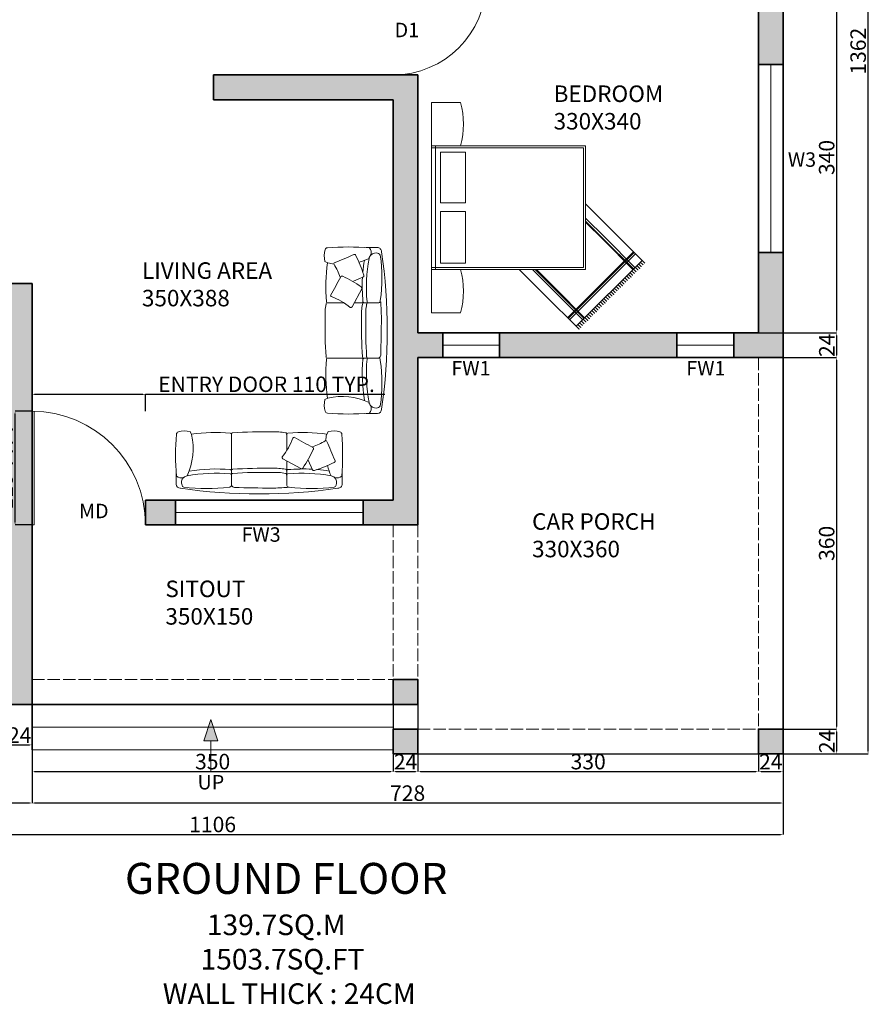
# Model space of a CAD drawing. Units: centimetres. Extents: x 2449 to 7478, y 778 to 2486.
# Tile 2 of 9: x 3072 to 3897, y 778 to 1732. Entities that reach past the tile are written whole.
import ezdxf

# ---------------------------------------------------------------- set-up
doc = ezdxf.new("R2010")
doc.units = ezdxf.units.CM
doc.linetypes.add('ACAD_ISO02W100', pattern=[15, 12, -3])
for name, color, linetype, lineweight in [('A-ANNO-DIMS', 2, 'Continuous', 18), ('A-ANNO-SYMB', 8, 'Continuous', 18), ('A-ANNO-TEXT', 7, 'Continuous', 18), ('A-ANNO-TITL', 7, 'Continuous', 25), ('A-AREA-IDEN', 7, 'Continuous', 18), ('A-COLS', 7, 'Continuous', 35), ('A-COLS-PATT', 7, 'Continuous', 13), ('A-DOOR', 4, 'Continuous', 18), ('A-FLOR', 7, 'Continuous', 25), ('A-FLOR-OVHD', 8, 'ACAD_ISO02W100', 18), ('A-FLOR-STRS', 7, 'Continuous', 18), ('A-WALL', 7, 'Continuous', 35), ('A-WALL-PATT', 7, 'Continuous', 13), ('B-FURNITURE', 22, 'Continuous', 18), ('Win', 1, 'Continuous', 18)]:
    doc.layers.add(name, color=color, linetype=linetype, lineweight=lineweight)
doc.styles.get("Standard").update_dxf_attribs({"font": 'arial.ttf'})
doc.dimstyles.new('ISO-25', dxfattribs={"dimtxt": 15, "dimasz": 2.5, "dimexe": 0, "dimexo": 0, "dimgap": 0, "dimtad": 1, "dimtxsty": 'Standard', "dimcen": 2.5, "dimadec": 0, "dimazin": 0, "dimtfac": 1, "dimtmove": 0, "dimatfit": 3, "dimfxl": 1, "dimarcsym": 0})

# ---------------------------------------------------------------- blocks, each defined once
blk = doc.blocks.new('ролар')
at = {"layer": 'B-FURNITURE'}
for p, q in [((182149, -12928), (182149, -13090)), ((182946, -12908), (182946, -13070)), ((183742, -12908), (183742, -13070)), ((184538, -12927), (184538, -13090)), ((182946, -13070), (182946, -13655)), ((183742, -13070), (183742, -13261)), ((183742, -13412), (183742, -13655))]:
    blk.add_line(p, q, dxfattribs=at)
blk.add_lwpolyline([(184124, -13426, 0.039108), (183972, -13160, 0.352413), (183942, -13151), (183685, -13293, 0.370087), (183675, -13320, -0.085318), (183831, -13592, 0.338149), (183848, -13604, -0.006963), (184118, -13456, 0.478074)], format="xyb", close=True, dxfattribs=at)
blk.add_lwpolyline([(184112, -13464, -0.054969), (184295, -13552, 0.338149), (184316, -13550, -0.006963), (184437, -13268, 0.478074), (184423, -13240, 0.039108), (184140, -13125, 0.352413), (184110, -13136), (184052, -13272)], format="xyb", dxfattribs=at)
for centre, radius, start, end in [((182209, -12928), 60, 90, 180), ((183344, -20690), 7904, 81.7476, 98.2524), ((182264, -12914), 28.1, 104.7154, 176.7534), ((182585, -15161), 2298, 81.7903, 98.2097), ((182918, -12915), 28.9, 15.2961, 99.1888), ((182999, -12942), 63.3, 99.7658, 147.0241), ((181568, 80195), 93085, 270.87421, 271.20678), ((183296, -20822), 7955, 86.6979, 88.3256), ((183770, -12915), 28.9, 80.8112, 164.7039), ((184102, -15161), 2298, 81.7903, 98.2097), ((184423, -12914), 28.1, 3.2466, 75.2846), ((184478, -12928), 60, 358.6006, 89.9879), ((182224, -13128), 110, 72.3508, 130.321), ((182322, -12954), 95.7, 154.4132, 226.8965), ((182340, -12922), 131, 230.7956, 255.727), ((184348, -12922), 131, 284.273, 309.2044), ((184365, -12954), 95.7, 313.1035, 25.5868), ((184464, -13128), 110, 49.679, 107.6492), ((186046, -13346), 3905, 175.5762, 184.4238), ((181452, -13440), 941, 347.608, 24.5904), ((182727, -10699), 2387, 259.8888, 274.8671), ((182725, -10712), 2434, 260.7796, 274.8194), ((182927, -13057), 20.3, 275.8765, 1.8), ((182927, -13117), 20.3, 275.8765, 1.8), ((182962, -13065), 17.3, 149.88, 272.0041), ((182962, -13125), 17.3, 149.88, 272.0041), ((183401, -6361), 6736, 266.2761, 271.089), ((183401, -6421), 6736, 266.2761, 271.089), ((183573, -12278), 819, 266.8813, 280.6931), ((183573, -12338), 819, 266.8813, 280.6931), ((183725, -13065), 17.3, 267.9959, 30.12), ((183725, -13125), 17.3, 267.9959, 30.12), ((183760, -13057), 20.3, 178.2, 264.1235), ((183760, -13117), 20.3, 178.2, 264.1235), ((183961, -10699), 2387, 265.1329, 280.1112), ((184001, -9721), 3425, 265.9379, 271.7664), ((184034, -11509), 1637, 275.2593, 281.2487), ((185235, -13440), 941, 155.4096, 164.8885), ((180641, -13346), 3905, 355.5762, 4.4238), ((185235, -13440), 941, 186.9661, 192.392), ((182195, -13642), 42.7, 187.075, 250.1971), ((182270, -13358), 336, 254.5718, 283.8571), ((181903, -13435), 512, 330.8359, 336.0732), ((182722, -11168), 2503, 261.8987, 274.7524), ((182927, -13643), 20.3, 275.8765, 1.8), ((182962, -13651), 17.3, 149.88, 272.0041), ((183401, -6946), 6736, 266.2761, 271.089), ((183573, -12863), 819, 266.8813, 280.6931), ((183725, -13651), 17.3, 267.9959, 30.12), ((183760, -13643), 20.3, 178.2, 264.1235), ((183966, -11168), 2503, 265.2476, 278.1013), ((184785, -13435), 512, 203.9268, 209.1641), ((184418, -13358), 336, 256.1429, 285.4282), ((184493, -13642), 42.7, 289.8029, 352.925)]:
    blk.add_arc(centre, radius, start, end, dxfattribs=at)
blk = doc.blocks.new('A$C376C2187')
at = {"layer": 'B-FURNITURE'}
for p, q in [((-1.53, 1.82), (-1.53, 2.24)), ((-1.53, 2.24), (-0.9, 2.24)), ((-0.9, 0), (-0.9, 2.24)), ((-0.9, 2.24), (0.9, 2.24)), ((-0.9, 2.24), (-0.9, 1.82)), ((-0.9, 2.182), (0.9, 2.182)), ((-0.87, 0.03), (-0.87, 2.24)), ((0.87, 2.24), (0.87, 0.03)), ((0.9, 2.24), (0.9, 0)), ((0.9, 1.82), (0.9, 2.24)), ((0.9, 2.24), (1.53, 2.24)), ((1.53, 2.24), (1.53, 1.82)), ((-0.807, 2.112), (-0.057, 2.112)), ((-0.807, 1.749), (-0.807, 2.112)), ((-0.057, 2.112), (-0.057, 1.749)), ((0.069, 2.112), (0.807, 2.112)), ((0.069, 2.112), (0.069, 1.749)), ((0.807, 2.112), (0.807, 1.749)), ((-0.807, 1.749), (-0.057, 1.749)), ((0.069, 1.749), (0.807, 1.749)), ((0.9, 0), (-0.9, 0)), ((0.87, 0.03), (-0.87, 0.03))]:
    blk.add_line(p, q, dxfattribs=at)
for centre in [(-1.215, 2.926), (1.215, 2.926)]:
    blk.add_arc(centre, 1.15, 254.0965, 285.9035, dxfattribs=at)
blk = doc.blocks.new('*D41')
at = {"layer": 'A-ANNO-DIMS', "color": 0, "lineweight": -2, "transparency": 16777216}
for p, q in [((3060.09, 1092.34), (3060.09, 1029.04)), ((3084.09, 1068.34), (3084.09, 1029.04)), ((3062.59, 1029.04), (3081.59, 1029.04))]:
    blk.add_line(p, q, dxfattribs=at)
at = {"layer": 'A-ANNO-DIMS', "color": 0, "transparency": 16777216}
for points in [[(3062.59, 1029.46), (3062.59, 1028.62), (3060.09, 1029.04)], [(3081.59, 1029.46), (3081.59, 1028.62), (3084.09, 1029.04)]]:
    blk.add_solid(points, dxfattribs=at)
at = {"layer": 'Defpoints', "color": 0, "transparency": 16777216}
for p in [(3060.09, 1092.34), (3084.09, 1068.34), (3084.09, 1029.04)]:
    blk.add_point(p, dxfattribs=at)
at = {"layer": 'A-ANNO-DIMS', "color": 0, "transparency": 16777216, "insert": (3072.09, 1036.57), "char_height": 15, "attachment_point": 5}
blk.add_mtext('24', dxfattribs=at)
blk = doc.blocks.new('*D42')
at = {"layer": 'A-ANNO-DIMS', "color": 0, "lineweight": -2, "transparency": 16777216}
for p, q in [((3084.09, 1024.34), (3084.09, 1003.23)), ((3434.09, 1020.34), (3434.09, 1003.23)), ((3086.59, 1003.23), (3431.59, 1003.23))]:
    blk.add_line(p, q, dxfattribs=at)
at = {"layer": 'A-ANNO-DIMS', "color": 0, "transparency": 16777216}
for points in [[(3086.59, 1003.64), (3086.59, 1002.81), (3084.09, 1003.23)], [(3431.59, 1003.64), (3431.59, 1002.81), (3434.09, 1003.23)]]:
    blk.add_solid(points, dxfattribs=at)
at = {"layer": 'Defpoints', "color": 0, "transparency": 16777216}
for p in [(3084.09, 1024.34), (3434.09, 1020.34), (3434.09, 1003.23)]:
    blk.add_point(p, dxfattribs=at)
at = {"layer": 'A-ANNO-DIMS', "color": 0, "transparency": 16777216, "insert": (3259.09, 1010.89), "char_height": 15, "attachment_point": 5}
blk.add_mtext('350', dxfattribs=at)
blk = doc.blocks.new('*D43')
at = {"layer": 'A-ANNO-DIMS', "color": 0, "lineweight": -2, "transparency": 16777216}
for p, q in [((3434.09, 1020.34), (3434.09, 1003.23)), ((3458.09, 1020.34), (3458.09, 1003.23)), ((3436.59, 1003.23), (3455.59, 1003.23))]:
    blk.add_line(p, q, dxfattribs=at)
at = {"layer": 'A-ANNO-DIMS', "color": 0, "transparency": 16777216}
for points in [[(3436.59, 1003.64), (3436.59, 1002.81), (3434.09, 1003.23)], [(3455.59, 1003.64), (3455.59, 1002.81), (3458.09, 1003.23)]]:
    blk.add_solid(points, dxfattribs=at)
at = {"layer": 'Defpoints', "color": 0, "transparency": 16777216}
for p in [(3434.09, 1020.34), (3458.09, 1020.34), (3458.09, 1003.23)]:
    blk.add_point(p, dxfattribs=at)
at = {"layer": 'A-ANNO-DIMS', "color": 0, "transparency": 16777216, "insert": (3446.09, 1010.76), "char_height": 15, "attachment_point": 5}
blk.add_mtext('24', dxfattribs=at)
blk = doc.blocks.new('*D44')
at = {"layer": 'A-ANNO-DIMS', "color": 0, "lineweight": -2, "transparency": 16777216}
for p, q in [((3458.09, 1020.34), (3458.09, 1003.23)), ((3788.09, 1020.34), (3788.09, 1003.23)), ((3460.59, 1003.23), (3785.59, 1003.23))]:
    blk.add_line(p, q, dxfattribs=at)
at = {"layer": 'A-ANNO-DIMS', "color": 0, "transparency": 16777216}
for points in [[(3460.59, 1003.64), (3460.59, 1002.81), (3458.09, 1003.23)], [(3785.59, 1003.64), (3785.59, 1002.81), (3788.09, 1003.23)]]:
    blk.add_solid(points, dxfattribs=at)
at = {"layer": 'Defpoints', "color": 0, "transparency": 16777216}
for p in [(3458.09, 1020.34), (3788.09, 1020.34), (3788.09, 1003.23)]:
    blk.add_point(p, dxfattribs=at)
at = {"layer": 'A-ANNO-DIMS', "color": 0, "transparency": 16777216, "insert": (3623.09, 1010.89), "char_height": 15, "attachment_point": 5}
blk.add_mtext('330', dxfattribs=at)
blk = doc.blocks.new('*D45')
at = {"layer": 'A-ANNO-DIMS', "color": 0, "lineweight": -2, "transparency": 16777216}
for p, q in [((3788.09, 1020.34), (3788.09, 1003.23)), ((3812.09, 1020.34), (3812.09, 1003.23)), ((3790.59, 1003.23), (3809.59, 1003.23))]:
    blk.add_line(p, q, dxfattribs=at)
at = {"layer": 'A-ANNO-DIMS', "color": 0, "transparency": 16777216}
for points in [[(3790.59, 1003.64), (3790.59, 1002.81), (3788.09, 1003.23)], [(3809.59, 1003.64), (3809.59, 1002.81), (3812.09, 1003.23)]]:
    blk.add_solid(points, dxfattribs=at)
at = {"layer": 'Defpoints', "color": 0, "transparency": 16777216}
for p in [(3788.09, 1020.34), (3812.09, 1020.34), (3812.09, 1003.23)]:
    blk.add_point(p, dxfattribs=at)
at = {"layer": 'A-ANNO-DIMS', "color": 0, "transparency": 16777216, "insert": (3800.09, 1010.76), "char_height": 15, "attachment_point": 5}
blk.add_mtext('24', dxfattribs=at)
blk = doc.blocks.new('*D51')
at = {"layer": 'A-ANNO-DIMS', "color": 0, "lineweight": -2, "transparency": 16777216}
for p, q in [((3788.09, 1768.34), (3863.83, 1768.34)), ((3863.83, 1765.84), (3863.83, 1430.84)), ((3788.09, 1428.34), (3863.83, 1428.34))]:
    blk.add_line(p, q, dxfattribs=at)
at = {"layer": 'A-ANNO-DIMS', "color": 0, "transparency": 16777216}
for points in [[(3863.42, 1765.84), (3864.25, 1765.84), (3863.83, 1768.34)], [(3863.42, 1430.84), (3864.25, 1430.84), (3863.83, 1428.34)]]:
    blk.add_solid(points, dxfattribs=at)
at = {"layer": 'Defpoints', "color": 0, "transparency": 16777216}
for p in [(3788.09, 1768.34), (3788.09, 1428.34), (3863.83, 1428.34)]:
    blk.add_point(p, dxfattribs=at)
at = {"layer": 'A-ANNO-DIMS', "color": 0, "transparency": 16777216, "insert": (3856.17, 1598.34), "char_height": 15, "attachment_point": 5, "rotation": 90}
blk.add_mtext('340', dxfattribs=at)
blk = doc.blocks.new('*D52')
at = {"layer": 'A-ANNO-DIMS', "color": 0, "lineweight": -2, "transparency": 16777216}
for p, q in [((3788.09, 1428.34), (3863.83, 1428.34)), ((3863.83, 1425.84), (3863.83, 1406.84)), ((3812.09, 1404.34), (3863.83, 1404.34))]:
    blk.add_line(p, q, dxfattribs=at)
at = {"layer": 'A-ANNO-DIMS', "color": 0, "transparency": 16777216}
for points in [[(3863.42, 1425.84), (3864.25, 1425.84), (3863.83, 1428.34)], [(3863.42, 1406.84), (3864.25, 1406.84), (3863.83, 1404.34)]]:
    blk.add_solid(points, dxfattribs=at)
at = {"layer": 'Defpoints', "color": 0, "transparency": 16777216}
for p in [(3788.09, 1428.34), (3812.09, 1404.34), (3863.83, 1404.34)]:
    blk.add_point(p, dxfattribs=at)
at = {"layer": 'A-ANNO-DIMS', "color": 0, "transparency": 16777216, "insert": (3856.3, 1416.34), "char_height": 15, "attachment_point": 5, "rotation": 90}
blk.add_mtext('24', dxfattribs=at)
blk = doc.blocks.new('*D53')
at = {"layer": 'A-ANNO-DIMS', "color": 0, "lineweight": -2, "transparency": 16777216}
for p, q in [((3812.09, 1404.34), (3863.83, 1404.34)), ((3863.83, 1401.84), (3863.83, 1046.84)), ((3812.09, 1044.34), (3863.83, 1044.34))]:
    blk.add_line(p, q, dxfattribs=at)
at = {"layer": 'A-ANNO-DIMS', "color": 0, "transparency": 16777216}
for points in [[(3863.42, 1401.84), (3864.25, 1401.84), (3863.83, 1404.34)], [(3863.42, 1046.84), (3864.25, 1046.84), (3863.83, 1044.34)]]:
    blk.add_solid(points, dxfattribs=at)
at = {"layer": 'Defpoints', "color": 0, "transparency": 16777216}
for p in [(3812.09, 1404.34), (3812.09, 1044.34), (3863.83, 1044.34)]:
    blk.add_point(p, dxfattribs=at)
at = {"layer": 'A-ANNO-DIMS', "color": 0, "transparency": 16777216, "insert": (3856.17, 1224.34), "char_height": 15, "attachment_point": 5, "rotation": 90}
blk.add_mtext('360', dxfattribs=at)
blk = doc.blocks.new('*D54')
at = {"layer": 'A-ANNO-DIMS', "color": 0, "lineweight": -2, "transparency": 16777216}
for p, q in [((3812.09, 1044.34), (3863.83, 1044.34)), ((3863.83, 1041.84), (3863.83, 1022.84)), ((3812.09, 1020.34), (3863.83, 1020.34))]:
    blk.add_line(p, q, dxfattribs=at)
at = {"layer": 'A-ANNO-DIMS', "color": 0, "transparency": 16777216}
for points in [[(3863.42, 1041.84), (3864.25, 1041.84), (3863.83, 1044.34)], [(3863.42, 1022.84), (3864.25, 1022.84), (3863.83, 1020.34)]]:
    blk.add_solid(points, dxfattribs=at)
at = {"layer": 'Defpoints', "color": 0, "transparency": 16777216}
for p in [(3812.09, 1044.34), (3812.09, 1020.34), (3863.83, 1020.34)]:
    blk.add_point(p, dxfattribs=at)
at = {"layer": 'A-ANNO-DIMS', "color": 0, "transparency": 16777216, "insert": (3856.3, 1032.34), "char_height": 15, "attachment_point": 5, "rotation": 90}
blk.add_mtext('24', dxfattribs=at)
blk = doc.blocks.new('*D55')
at = {"layer": 'A-ANNO-DIMS', "color": 0, "lineweight": -2, "transparency": 16777216}
for p, q in [((3084.09, 1068.34), (3084.09, 972.69)), ((3812.09, 1020.34), (3812.09, 972.69)), ((3809.59, 972.69), (3086.59, 972.69))]:
    blk.add_line(p, q, dxfattribs=at)
at = {"layer": 'A-ANNO-DIMS', "color": 0, "transparency": 16777216}
for points in [[(3086.59, 973.11), (3086.59, 972.27), (3084.09, 972.69)], [(3809.59, 973.11), (3809.59, 972.27), (3812.09, 972.69)]]:
    blk.add_solid(points, dxfattribs=at)
at = {"layer": 'Defpoints', "color": 0, "transparency": 16777216}
for p in [(3084.09, 1068.34), (3812.09, 1020.34), (3084.09, 972.69)]:
    blk.add_point(p, dxfattribs=at)
at = {"layer": 'A-ANNO-DIMS', "color": 0, "transparency": 16777216, "insert": (3448.09, 980.35), "char_height": 15, "attachment_point": 5}
blk.add_mtext('728', dxfattribs=at)
blk = doc.blocks.new('*D56')
at = {"layer": 'A-ANNO-DIMS', "color": 0, "lineweight": -2, "transparency": 16777216}
for p, q in [((2706.09, 1068.34), (2706.09, 972.69)), ((3084.09, 1068.34), (3084.09, 972.69)), ((3081.59, 972.69), (2708.59, 972.69))]:
    blk.add_line(p, q, dxfattribs=at)
at = {"layer": 'A-ANNO-DIMS', "color": 0, "transparency": 16777216}
for points in [[(2708.59, 973.11), (2708.59, 972.27), (2706.09, 972.69)], [(3081.59, 973.11), (3081.59, 972.27), (3084.09, 972.69)]]:
    blk.add_solid(points, dxfattribs=at)
at = {"layer": 'Defpoints', "color": 0, "transparency": 16777216}
for p in [(2706.09, 1068.34), (3084.09, 1068.34), (2706.09, 972.69)]:
    blk.add_point(p, dxfattribs=at)
at = {"layer": 'A-ANNO-DIMS', "color": 0, "transparency": 16777216, "insert": (2895.09, 980.35), "char_height": 15, "attachment_point": 5}
blk.add_mtext('378', dxfattribs=at)
blk = doc.blocks.new('*D57')
at = {"layer": 'A-ANNO-DIMS', "color": 0, "lineweight": -2, "transparency": 16777216}
for p, q in [((2706.09, 1068.34), (2706.09, 942.3)), ((3812.09, 1044.34), (3812.09, 942.3)), ((2708.59, 942.3), (3809.59, 942.3))]:
    blk.add_line(p, q, dxfattribs=at)
at = {"layer": 'A-ANNO-DIMS', "color": 0, "transparency": 16777216}
for points in [[(2708.59, 942.72), (2708.59, 941.88), (2706.09, 942.3)], [(3809.59, 942.72), (3809.59, 941.88), (3812.09, 942.3)]]:
    blk.add_solid(points, dxfattribs=at)
at = {"layer": 'Defpoints', "color": 0, "transparency": 16777216}
for p in [(2706.09, 1068.34), (3812.09, 1044.34), (3812.09, 942.3)]:
    blk.add_point(p, dxfattribs=at)
at = {"layer": 'A-ANNO-DIMS', "color": 0, "transparency": 16777216, "insert": (3259.09, 949.96), "char_height": 15, "attachment_point": 5}
blk.add_mtext('1106', dxfattribs=at)
blk = doc.blocks.new('*D58')
at = {"layer": 'A-ANNO-DIMS', "color": 0, "lineweight": -2, "transparency": 16777216}
for p, q in [((3812.09, 2382.34), (3894.34, 2382.34)), ((3894.34, 1022.84), (3894.34, 2379.84)), ((3812.09, 1020.34), (3894.34, 1020.34))]:
    blk.add_line(p, q, dxfattribs=at)
at = {"layer": 'A-ANNO-DIMS', "color": 0, "transparency": 16777216}
for points in [[(3893.92, 2379.84), (3894.76, 2379.84), (3894.34, 2382.34)], [(3893.92, 1022.84), (3894.76, 1022.84), (3894.34, 1020.34)]]:
    blk.add_solid(points, dxfattribs=at)
at = {"layer": 'Defpoints', "color": 0, "transparency": 16777216}
for p in [(3812.09, 2382.34), (3894.34, 2382.34), (3812.09, 1020.34)]:
    blk.add_point(p, dxfattribs=at)
at = {"layer": 'A-ANNO-DIMS', "color": 0, "transparency": 16777216, "insert": (3886.68, 1701.34), "char_height": 15, "attachment_point": 5, "rotation": 90}
blk.add_mtext('1362', dxfattribs=at)
blk = doc.blocks.new('1')
for p, q in [((5854.12, 1703.75), (5854.12, 1593.75)), ((5856.12, 1703.75), (5856.12, 1593.75)), ((5856.12, 1593.75), (5854.12, 1593.75))]:
    blk.add_line(p, q)
blk.add_arc((5854.12, 1593.75), 110, 0, 90)
blk = doc.blocks.new('2')
for p, q in [((5717.35, 1812.71), (5717.35, 1722.71)), ((5719.35, 1812.71), (5719.35, 1722.71)), ((5719.35, 1722.71), (5717.35, 1722.71))]:
    blk.add_line(p, q)
blk.add_arc((5717.35, 1722.71), 90, 0, 90)
blk = doc.blocks.new('RUG-FRINGED-B')
for p, q in [((90.45, 95.22), (64.35, 121.32)), ((64.35, 107.43), (83.5, 88.28)), ((64.35, 104.72), (82.15, 86.92)), ((64.35, 103.56), (81.57, 86.34)), ((110.18, 57.73), (81.57, 86.34)), ((110.76, 58.31), (82.15, 86.92)), ((112.12, 59.66), (83.5, 88.28)), ((90.45, 95.22), (119.07, 66.61)), ((110.74, 74.93), (46.79, 10.99)), ((111.32, 74.35), (47.37, 10.4)), ((112.68, 73), (48.73, 9.05)), ((0, 57.78), (26.5, 31.28)), ((32.89, 37.67), (12.78, 57.78)), ((34.25, 39.02), (15.49, 57.78)), ((34.83, 39.6), (16.65, 57.78)), ((119.07, 66.61), (55.12, 2.66)), ((110.66, 58.21), (113.29, 55.58)), ((112.34, 59.89), (114.97, 57.26)), ((114.02, 61.57), (116.65, 58.94)), ((115.7, 63.25), (118.33, 60.62)), ((117.39, 64.93), (120.01, 62.3)), ((119.07, 66.61), (121.69, 63.98)), ((100.58, 48.13), (103.21, 45.5)), ((102.26, 49.81), (104.89, 47.18)), ((103.94, 51.49), (106.57, 48.86)), ((105.62, 53.17), (108.25, 50.54)), ((107.3, 54.85), (109.93, 52.22)), ((108.98, 56.53), (111.61, 53.9)), ((34.25, 39.02), (62.86, 10.4)), ((34.83, 39.6), (63.44, 10.99)), ((92.18, 39.73), (94.81, 37.1)), ((93.86, 41.41), (96.49, 38.78)), ((95.54, 43.09), (98.17, 40.46)), ((97.22, 44.77), (99.85, 42.14)), ((98.9, 46.45), (101.53, 43.82)), ((55.12, 2.66), (26.5, 31.28)), ((32.89, 37.67), (61.51, 9.05)), ((82.1, 29.65), (84.73, 27.02)), ((83.78, 31.33), (86.41, 28.7)), ((85.46, 33.01), (88.09, 30.38)), ((87.14, 34.69), (89.77, 32.06)), ((88.82, 36.37), (91.45, 33.74)), ((90.5, 38.05), (93.13, 35.42)), ((72.02, 19.57), (74.65, 16.94)), ((73.7, 21.25), (76.33, 18.62)), ((75.38, 22.93), (78.01, 20.3)), ((77.06, 24.61), (79.69, 21.98)), ((78.74, 26.29), (81.37, 23.66)), ((80.42, 27.97), (83.05, 25.34)), ((63.62, 11.17), (66.25, 8.54)), ((65.3, 12.85), (67.93, 10.22)), ((66.98, 14.53), (69.61, 11.9)), ((68.66, 16.21), (71.29, 13.58)), ((70.34, 17.89), (72.97, 15.26)), ((55.22, 2.76), (57.85, 0.14)), ((56.9, 4.44), (59.53, 1.82)), ((58.58, 6.12), (61.21, 3.5)), ((60.26, 7.8), (62.89, 5.18)), ((61.94, 9.48), (64.57, 6.86))]:
    blk.add_line(p, q)
for centre in [(115.03, 57.2), (116.71, 58.88), (118.39, 60.56), (120.07, 62.24), (121.75, 63.92), (106.63, 48.8), (108.31, 50.48), (109.99, 52.16), (111.67, 53.84), (113.35, 55.52), (96.55, 38.72), (98.23, 40.4), (99.91, 42.08), (101.59, 43.76), (103.27, 45.44), (104.95, 47.12), (86.47, 28.64), (88.15, 30.32), (89.83, 32), (91.51, 33.68), (93.19, 35.36), (94.87, 37.04), (78.07, 20.24), (79.75, 21.92), (81.43, 23.6), (83.11, 25.28), (84.79, 26.96), (67.99, 10.16), (69.67, 11.84), (71.35, 13.52), (73.03, 15.2), (74.71, 16.88), (76.39, 18.56), (57.91, 0.08), (59.59, 1.76), (61.27, 3.44), (62.95, 5.12), (64.63, 6.8), (66.31, 8.48)]:
    blk.add_circle(centre, 0.0789)
blk = doc.blocks.new('ARROW-ENTRY-UP')
at = {"transparency": 33554687}
h = blk.add_hatch(color=256, dxfattribs=at)
h.dxf.hatch_style = 1
h.paths.add_polyline_path([(-6.84, 30.34), (6.84, 30.34), (0, 51.25)])
blk.add_line((0, 30.34), (0, 0))
blk.add_lwpolyline([(0, 51.25), (-6.84, 30.34), (6.84, 30.34)], close=True)
blk = doc.blocks.new('*D72')
at = {"layer": 'A-ANNO-DIMS', "color": 0, "lineweight": -2, "transparency": 16777216}
for p, q in [((3084.09, 1352.34), (3084.09, 1368.84)), ((3086.59, 1368.84), (3191.59, 1368.84)), ((3194.09, 1352.34), (3194.09, 1368.84)), ((3194.09, 1368.84), (3426, 1368.84))]:
    blk.add_line(p, q, dxfattribs=at)
at = {"layer": 'A-ANNO-DIMS', "color": 0, "transparency": 16777216}
for points in [[(3086.59, 1369.26), (3086.59, 1368.42), (3084.09, 1368.84)], [(3191.59, 1369.26), (3191.59, 1368.42), (3194.09, 1368.84)]]:
    blk.add_solid(points, dxfattribs=at)
at = {"layer": 'Defpoints', "color": 0, "transparency": 16777216}
for p in [(3194.09, 1368.84), (3084.09, 1352.34), (3194.09, 1352.34)]:
    blk.add_point(p, dxfattribs=at)
at = {"layer": 'A-ANNO-DIMS', "color": 0, "transparency": 16777216, "insert": (3311.29, 1376.6), "char_height": 15, "attachment_point": 5}
blk.add_mtext('ENTRY DOOR 110 TYP.', dxfattribs=at)
blk = doc.blocks.new('*D73')
at = {"layer": 'A-ANNO-DIMS', "color": 0, "lineweight": -2, "transparency": 16777216}
for p, q in [((3084.09, 1352.34), (3067.59, 1352.34)), ((3067.59, 1244.84), (3067.59, 1349.84)), ((3084.09, 1242.34), (3067.59, 1242.34))]:
    blk.add_line(p, q, dxfattribs=at)
at = {"layer": 'A-ANNO-DIMS', "color": 0, "transparency": 16777216}
for points in [[(3067.17, 1349.84), (3068, 1349.84), (3067.59, 1352.34)], [(3067.17, 1244.84), (3068, 1244.84), (3067.59, 1242.34)]]:
    blk.add_solid(points, dxfattribs=at)
at = {"layer": 'Defpoints', "color": 0, "transparency": 16777216}
for p in [(3067.59, 1352.34), (3084.09, 1352.34), (3084.09, 1242.34)]:
    blk.add_point(p, dxfattribs=at)
at = {"layer": 'A-ANNO-DIMS', "color": 0, "transparency": 16777216, "insert": (3059.93, 1297.34), "char_height": 15, "attachment_point": 5, "rotation": 90}
blk.add_mtext('110 TYP.', dxfattribs=at)

msp = doc.modelspace()

# ---------------------------------------------------------------- hatches: boundary and pattern name
at = {"layer": 'A-COLS-PATT'}
h = msp.add_hatch(color=256, dxfattribs=at)
h.dxf.hatch_style = 1
h.paths.add_polyline_path([(3458.088, 1092.34), (3434.088, 1092.34), (3434.088, 1068.34), (3458.088, 1068.34)])
h = msp.add_hatch(color=256, dxfattribs=at)
h.dxf.hatch_style = 1
h.paths.add_polyline_path([(3434.088, 1020.34), (3458.088, 1020.34), (3458.088, 1044.34), (3434.088, 1044.34)])
h = msp.add_hatch(color=256, dxfattribs=at)
h.dxf.hatch_style = 1
h.paths.add_polyline_path([(3788.088, 1020.34), (3812.088, 1020.34), (3812.088, 1044.34), (3788.088, 1044.34)])
at = {"layer": 'A-WALL-PATT'}
h = msp.add_hatch(color=256, dxfattribs=at)
h.dxf.hatch_style = 1
h.paths.add_polyline_path([(3060.088, 1092.34), (2986.088, 1092.34), (2986.088, 1068.34), (3084.088, 1068.34), (3084.088, 1476.34), (3060.088, 1476.34)])
h.paths.add_polyline_path([(2706.088, 1167.34), (2730.088, 1167.34), (2730.088, 1377.34), (2706.088, 1377.34)])
h.paths.add_polyline_path([(2804.088, 1068.34), (2804.088, 1092.34), (2730.088, 1092.34), (2730.088, 1112.34), (2706.088, 1112.34), (2706.088, 1068.34)])
h.paths.add_polyline_path([(2730.088, 1551.34), (2706.088, 1551.34), (2706.088, 1432.34), (2730.088, 1432.34), (2730.088, 1452.34), (2970.088, 1452.34), (2970.088, 1476.34), (2730.088, 1476.34)])
h.paths.add_polyline_path([(3434.088, 1654.34), (3434.088, 1266.34), (3405.088, 1266.34), (3405.088, 1242.34), (3458.088, 1242.34), (3458.088, 1404.34), (3482.088, 1404.34), (3482.088, 1428.34), (3458.088, 1428.34), (3458.088, 1678.34), (3260.088, 1678.34), (3260.088, 1654.34)])
h.paths.add_polyline_path([(3223.088, 1266.34), (3194.088, 1266.34), (3194.088, 1242.34), (3223.088, 1242.34)])
h.paths.add_polyline_path([(3812.088, 1506.339), (3788.088, 1506.339), (3788.088, 1428.34), (3764.088, 1428.34), (3764.088, 1404.34), (3812.088, 1404.34)])
h.paths.add_polyline_path([(3709.088, 1404.34), (3709.088, 1428.34), (3537.088, 1428.34), (3537.088, 1404.34)])
h.paths.add_polyline_path([(3788.088, 1688.339), (3812.088, 1688.339), (3812.088, 1826.34), (3788.088, 1826.34), (3788.088, 1792.34), (3647.088, 1792.34), (3647.088, 1768.34), (3788.088, 1768.34)])
h.paths.add_polyline_path([(3788.088, 1956.34), (3548.088, 1956.34), (3548.088, 1792.34), (3434.088, 1792.34), (3434.088, 1768.34), (3572.088, 1768.34), (3572.088, 1932.34), (3788.088, 1932.34), (3788.088, 1898.34), (3812.088, 1898.34), (3812.088, 2065.339), (3788.088, 2065.339)])
h.paths.add_polyline_path([(3788.088, 2358.34), (3788.088, 2247.339), (3812.088, 2247.339), (3812.088, 2382.34), (3764.088, 2382.34), (3764.088, 2358.34)])
h.paths.add_polyline_path([(3537.088, 2382.34), (3537.088, 2358.34), (3709.088, 2358.34), (3709.088, 2382.34)])
h.paths.add_polyline_path([(3458.088, 2358.34), (3482.088, 2358.34), (3482.088, 2382.34), (3434.088, 2382.34), (3434.088, 2214.34), (3395.088, 2214.34), (3395.088, 2190.34), (3434.088, 2190.34), (3434.088, 2065.34), (3458.088, 2065.34)])
h.paths.add_polyline_path([(3231.088, 2214.34), (3231.088, 2190.34), (3260.088, 2190.34), (3260.088, 1966.34), (3434.088, 1966.34), (3434.088, 1932.34), (3458.088, 1932.34), (3458.088, 1990.34), (3284.088, 1990.34), (3284.088, 2190.34), (3323.088, 2190.34), (3323.088, 2214.34)])
h.paths.add_polyline_path([(3130.088, 2190.34), (3159.088, 2190.34), (3159.088, 2214.34), (3032.088, 2214.34), (3032.088, 2190.34), (3106.088, 2190.34), (3106.088, 1836.34), (3130.088, 1836.34), (3130.088, 1966.34), (3185.088, 1966.34), (3185.088, 1990.34), (3130.088, 1990.34)])
h.paths.add_polyline_path([(2738.088, 2214.34), (2738.088, 2190.34), (2752.088, 2190.34), (2752.088, 1935.34), (2776.088, 1935.34), (2776.088, 2190.34), (2850.088, 2190.34), (2850.088, 2214.34)])
h.paths.add_polyline_path([(2578.088, 2152.839), (2602.088, 2152.839), (2602.088, 2190.34), (2616.088, 2190.34), (2616.088, 2214.34), (2578.088, 2214.34)])
h.paths.add_polyline_path([(2578.088, 1935.34), (2602.088, 1935.34), (2602.088, 1970.839), (2578.088, 1970.839)])
h.paths.add_polyline_path([(2706.088, 1836.34), (2706.088, 1791.34), (2730.088, 1791.34), (2730.088, 1836.34), (3016.088, 1836.34), (3016.088, 1860.34), (2578.088, 1860.34), (2578.088, 1836.34)])

# ---------------------------------------------------------------- linework, layer by layer
at = {"layer": 'A-COLS'}
for points in [[(3434.088, 1068.34), (3458.088, 1068.34), (3458.088, 1092.34), (3434.088, 1092.34)], [(3434.088, 1020.34), (3458.088, 1020.34), (3458.088, 1044.34), (3434.088, 1044.34)], [(3788.088, 1020.34), (3812.088, 1020.34), (3812.088, 1044.34), (3788.088, 1044.34)]]:
    msp.add_lwpolyline(points, close=True, dxfattribs=at)
at = {"layer": 'A-FLOR'}
for p, q in [((3434.088, 1092.34), (3434.088, 1020.34)), ((3458.088, 1092.34), (3458.088, 1044.34)), ((3434.088, 1044.34), (3458.088, 1044.34)), ((3434.088, 1020.34), (3812.088, 1020.34))]:
    msp.add_line(p, q, dxfattribs=at)
at = {"layer": 'A-FLOR-OVHD'}
for p, q in [((3788.088, 1404.34), (3788.088, 1044.34)), ((3434.088, 1242.34), (3434.088, 1092.34)), ((3458.088, 1242.34), (3458.088, 1092.34)), ((3084.088, 1092.34), (3458.088, 1092.34)), ((3458.088, 1044.34), (3788.088, 1044.34))]:
    msp.add_line(p, q, dxfattribs=at)
at = {"layer": 'A-FLOR-STRS'}
for p, q in [((3084.088, 1046.34), (3434.088, 1046.34)), ((3084.088, 1024.34), (3434.088, 1024.34))]:
    msp.add_line(p, q, dxfattribs=at)
at = {"layer": 'A-WALL'}
for p, q in [((3812.088, 2382.34), (3812.088, 1020.34)), ((3788.088, 1768.34), (3788.088, 1428.34)), ((3788.088, 1688.339), (3812.088, 1688.339)), ((3260.088, 1678.34), (3458.088, 1678.34)), ((3260.088, 1678.34), (3260.088, 1654.34)), ((3458.088, 1678.34), (3458.088, 1428.34)), ((3260.088, 1654.34), (3434.088, 1654.34)), ((3434.088, 1654.34), (3434.088, 1266.34)), ((3788.088, 1506.339), (3812.088, 1506.339)), ((3060.088, 1476.34), (3084.088, 1476.34)), ((3084.088, 1476.34), (3084.088, 1024.34)), ((3458.088, 1428.34), (3788.088, 1428.34)), ((3482.088, 1428.34), (3482.088, 1404.34)), ((3537.088, 1428.34), (3537.088, 1404.34)), ((3709.088, 1428.34), (3709.088, 1404.34)), ((3764.088, 1428.34), (3764.088, 1404.34)), ((3458.088, 1404.34), (3812.088, 1404.34)), ((3458.088, 1404.34), (3458.088, 1242.34)), ((3194.088, 1266.34), (3194.088, 1242.34)), ((3194.088, 1266.34), (3434.088, 1266.34)), ((3223.088, 1266.34), (3223.088, 1242.34)), ((3405.088, 1266.34), (3405.088, 1242.34)), ((3194.088, 1242.34), (3458.088, 1242.34)), ((2706.088, 1068.34), (3458.088, 1068.34))]:
    msp.add_line(p, q, dxfattribs=at)
at = {"layer": 'Win'}
for p, q in [((3800.088, 1688.339), (3800.088, 1506.339)), ((3482.088, 1416.34), (3537.088, 1416.34)), ((3709.088, 1416.34), (3764.088, 1416.34)), ((3223.088, 1254.34), (3405.088, 1254.34))]:
    msp.add_line(p, q, dxfattribs=at)

# ---------------------------------------------------------------- block references
at = {"layer": 'A-ANNO-SYMB'}
msp.add_blockref('ARROW-ENTRY-UP', (3257.361, 1002.514), dxfattribs=at)
at = {"layer": 'A-DOOR', "rotation": 270}
msp.add_blockref('2', (1711.374, 7485.689), dxfattribs=at)
at = {"layer": 'A-DOOR'}
msp.add_blockref('1', (-2770.032, -351.413), dxfattribs=at)
at = {"layer": 'B-FURNITURE'}
for name, p, xscale, yscale, zscale, rotation in [('A$C376C2187', (3620.579, 1549.792), 66.63496932822166, 66.63496932822166, 66.63496932822166, 90), ('ролар', (4288.997, -10910.435), -0.0673113048210398, 0.0673113048210398, 0.0673113048210398, 270), ('ролар', (-9036.952, 411.556), -0.0673113048210398, 0.0673113048210398, 0.0673113048210398, 180)]:
    msp.add_blockref(name, p, dxfattribs=dict(at, xscale=xscale, yscale=yscale, zscale=zscale, rotation=rotation))
msp.add_blockref('RUG-FRINGED-B', (3556.226, 1432.041), dxfattribs=at)

# ---------------------------------------------------------------- texts
at = {"layer": 'A-ANNO-TEXT', "char_height": 14, "attachment_point": 1}
for s, insert in [('{\\fTimes New Roman|b0|i0|c0|p18;\\PD1}', (3435.478, 1752.244)), ('{\\fTimes New Roman|b0|i0|c0|p18;\\PW3}', (3816.594, 1626.636)), ('{\\fTimes New Roman|b0|i0|c0|p18;\\PFW1}', (3490.53, 1424.402)), ('{\\fTimes New Roman|b0|i0|c0|p18;\\PFW1}', (3718.201, 1424.402)), ('{\\fTimes New Roman|b0|i0|c0|p18;\\PMD}', (3129.638, 1286.053)), ('{\\fTimes New Roman|b0|i0|c0|p18;\\PFW3}', (3287.102, 1263.247)), ('{\\fTimes New Roman|b0|i0|c0|p18;\\PUP}', (3244.454, 1023.213))]:
    msp.add_mtext_dynamic_manual_height_columns(s, width=211.90348, gutter_width=12.5, heights=[0], dxfattribs=dict(at, insert=insert))
at = {"layer": 'A-ANNO-TITL', "insert": (3174.092, 914.668), "char_height": 30, "attachment_point": 1}
msp.add_mtext_dynamic_manual_height_columns('{\\fTimes New Roman|b0|i0|c0|p18;GROUND FLOOR\\P\\H0.66667x;             139.7SQ.M\\P            1503.7SQ.FT\\P      WALL THICK : 24CM}', width=483.87687, gutter_width=12.5, heights=[0], dxfattribs=at)
at = {"layer": 'A-AREA-IDEN', "char_height": 16, "attachment_point": 1}
for s, insert in [('{\\fTimes New Roman|b0|i0|c0|p18;\\PBEDROOM           330X340}', (3589.586, 1694.796)), ('{\\fTimes New Roman|b0|i0|c0|p18;\\PLIVING AREA             350X388}', (3190.569, 1523.391)), ('{\\fTimes New Roman|b0|i0|c0|p18;\\PCAR PORCH  330X360}', (3568.713, 1280.209)), ('{\\fTimes New Roman|b0|i0|c0|p18;\\PSITOUT           350X150}', (3213.304, 1214.933))]:
    msp.add_mtext_dynamic_manual_height_columns(s, width=211.90348, gutter_width=12.5, heights=[0], dxfattribs=dict(at, insert=insert))

# ---------------------------------------------------------------- dimensions: what is measured, and where the dimension line sits
at = {"layer": 'A-ANNO-DIMS'}
for base, p1, p2, override, picture, middle in [((3894.34, 2382.34), (3812.088, 1020.34), (3812.088, 2382.34), {"dimclrd": 0, "dimclre": 0, "dimclrt": 0}, '*D58', (3886.676, 1701.34)), ((3863.835, 1428.34), (3788.088, 1768.34), (3788.088, 1428.34), {"dimclrd": 0, "dimclre": 0, "dimclrt": 0, "dimtmove": 1}, '*D51', (3856.171, 1598.34)), ((3863.835, 1404.34), (3788.088, 1428.34), (3812.088, 1404.34), {"dimclrd": 0, "dimclre": 0, "dimclrt": 0, "dimtmove": 1}, '*D52', (3856.304, 1416.34)), ((3863.835, 1044.34), (3812.088, 1404.34), (3812.088, 1044.34), {"dimclrd": 0, "dimclre": 0, "dimclrt": 0, "dimtmove": 1}, '*D53', (3856.171, 1224.34)), ((3863.835, 1020.34), (3812.088, 1044.34), (3812.088, 1020.34), {"dimclrd": 0, "dimclre": 0, "dimclrt": 0, "dimtmove": 1}, '*D54', (3856.304, 1032.34))]:
    dim = msp.add_linear_dim(base=base, p1=p1, p2=p2, angle=90, dimstyle='ISO-25', override=override, dxfattribs=at)
    dim.commit()
    dim.dimension.update_dxf_attribs({"geometry": picture, "text_midpoint": middle})
dim = msp.add_linear_dim(base=(3194.088, 1368.84), p1=(3084.088, 1352.34), p2=(3194.088, 1352.34), text='ENTRY DOOR <> TYP.', dimstyle='ISO-25', override={"dimdec": 0, "dimlfac": 1, "dimrnd": 0, "dimzin": 0, "dimdsep": 46, "dimlunit": 2}, dxfattribs=at)
dim.commit()
dim.dimension.update_dxf_attribs({"geometry": '*D72', "text_midpoint": (3311.293, 1376.601)})
dim = msp.add_linear_dim(base=(3067.588, 1352.34), p1=(3084.088, 1242.34), p2=(3084.088, 1352.34), angle=90, text='<> TYP.', dimstyle='ISO-25', override={"dimdec": 0, "dimlfac": 1, "dimrnd": 0, "dimzin": 0, "dimdsep": 46, "dimlunit": 2}, dxfattribs=at)
dim.commit()
dim.dimension.update_dxf_attribs({"geometry": '*D73', "text_midpoint": (3059.93, 1297.34)})
for base, p1, p2, override, picture, middle in [((3084.088, 1029.039), (3060.088, 1092.34), (3084.088, 1068.34), {"dimclrd": 0, "dimclre": 0, "dimclrt": 0, "dimtmove": 1}, '*D41', (3072.088, 1036.569)), ((2706.088, 972.69), (3084.088, 1068.34), (2706.088, 1068.34), {"dimclrd": 0, "dimclre": 0, "dimclrt": 0, "dimtmove": 1}, '*D56', (2895.088, 980.354)), ((3812.088, 942.302), (2706.088, 1068.34), (3812.088, 1044.34), {"dimclrd": 0, "dimclre": 0, "dimclrt": 0}, '*D57', (3259.088, 949.96)), ((3084.088, 972.69), (3812.088, 1020.34), (3084.088, 1068.34), {"dimclrd": 0, "dimclre": 0, "dimclrt": 0}, '*D55', (3448.088, 980.349)), ((3434.088, 1003.227), (3084.088, 1024.34), (3434.088, 1020.34), {"dimclrd": 0, "dimclre": 0, "dimclrt": 0}, '*D42', (3259.088, 1010.891)), ((3458.088, 1003.227), (3434.088, 1020.34), (3458.088, 1020.34), {"dimclrd": 0, "dimclre": 0, "dimclrt": 0, "dimtmove": 1}, '*D43', (3446.088, 1010.758)), ((3788.088, 1003.227), (3458.088, 1020.34), (3788.088, 1020.34), {"dimclrd": 0, "dimclre": 0, "dimclrt": 0, "dimtmove": 1}, '*D44', (3623.088, 1010.891)), ((3812.088, 1003.227), (3788.088, 1020.34), (3812.088, 1020.34), {"dimclrd": 0, "dimclre": 0, "dimclrt": 0, "dimtmove": 1}, '*D45', (3800.088, 1010.758))]:
    dim = msp.add_linear_dim(base=base, p1=p1, p2=p2, dimstyle='ISO-25', override=override, dxfattribs=at)
    dim.commit()
    dim.dimension.update_dxf_attribs({"geometry": picture, "text_midpoint": middle})

doc.saveas('drawing.dxf')
